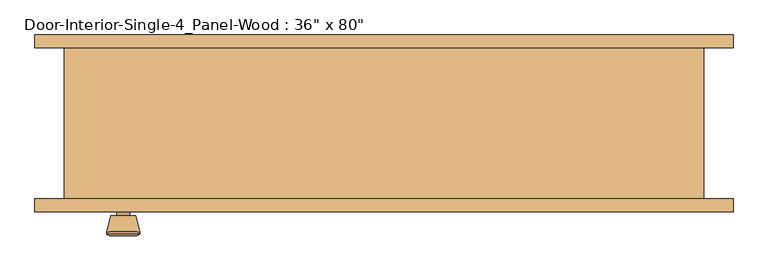
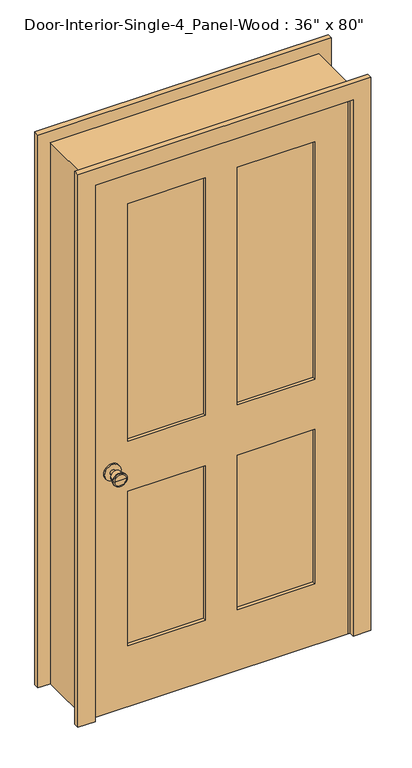
"""IFC4 building model written with IfcOpenShell, lengths in millimetres: door geometry."""

from ifc_helpers import new_model, si_unit, point, frame, frame_2d, origin, place, context, project, spatial, polyline, circle_curve, trimmed, segment, composite_curve, outline, extrude, faceted_brep, source, transform, mapped, element, save
from ifc_brep_helpers import plane_surface, cylinder_surface, revolved_surface, advanced_brep


def door_4c85932b(model_context):
    return source(origin(), model_context, "Body", "SolidModel", [
        advanced_brep(
        [(-393.7, -70.2, 914.4), (-403.7, -70.2, 914.4), (-383.7, -70.2, 914.4), (-373.2241324, -21.2, 914.4), (-414.1758676, -21.2, 914.4), (-393.7, -21.2, 914.4), (-368.7, -23.0278681, 914.4), (-418.7, -23.0278681, 914.4), (-368.7, -26.4915463, 914.4), (-418.7, -26.4915463, 914.4), (-375.063764, -51.2, 914.4), (-412.336236, -51.2, 914.4), (-383.7, -51.2, 914.4), (-403.7, -51.2, 914.4)],
        [
            (0, 1),
            (1, 2, circle_curve(frame((-393.7, -70.2, 914.4), z_axis=(0.0, -1.0, 0.0), x_axis=(-1.0, 0.0, 0.0)), 10.0)),
            (2, 0),
            (2, 1, circle_curve(frame((-393.7, -70.2, 914.4), z_axis=(0.0, -1.0, 0.0), x_axis=(-1.0, 0.0, 0.0)), 10.0)),
            (3, 4, circle_curve(frame((-393.7, -21.2, 914.4), z_axis=(0.0, 1.0, 0.0), x_axis=(-1.0, 0.0, 0.0)), 20.4758676)),
            (4, 5),
            (5, 3),
            (4, 3, circle_curve(frame((-393.7, -21.2, 914.4), z_axis=(0.0, 1.0, 0.0), x_axis=(-1.0, 0.0, 0.0)), 20.4758676)),
            (6, 7, circle_curve(frame((-393.7, -23.0278681, 914.4), z_axis=(0.0, 1.0, 0.0), x_axis=(-1.0, 0.0, 0.0)), 25.0)),
            (7, 4),
            (3, 6),
            (7, 6, circle_curve(frame((-393.7, -23.0278681, 914.4), z_axis=(0.0, 1.0, 0.0), x_axis=(-1.0, 0.0, 0.0)), 25.0)),
            (8, 9, circle_curve(frame((-393.7, -26.4915463, 914.4), z_axis=(0.0, 1.0, 0.0), x_axis=(-1.0, 0.0, 0.0)), 25.0)),
            (9, 7),
            (6, 8),
            (9, 8, circle_curve(frame((-393.7, -26.4915463, 914.4), z_axis=(0.0, 1.0, 0.0), x_axis=(-1.0, 0.0, 0.0)), 25.0)),
            (10, 11, circle_curve(frame((-393.7, -51.2, 914.4), z_axis=(0.0, 1.0, 0.0), x_axis=(-1.0, 0.0, 0.0)), 18.636236)),
            (11, 9),
            (8, 10),
            (11, 10, circle_curve(frame((-393.7, -51.2, 914.4), z_axis=(0.0, 1.0, 0.0), x_axis=(-1.0, 0.0, 0.0)), 18.636236)),
            (12, 13, circle_curve(frame((-393.7, -51.2, 914.4), z_axis=(0.0, 1.0, 0.0), x_axis=(-1.0, 0.0, 0.0)), 10.0)),
            (13, 11),
            (10, 12),
            (13, 12, circle_curve(frame((-393.7, -51.2, 914.4), z_axis=(0.0, 1.0, 0.0), x_axis=(-1.0, 0.0, 0.0)), 10.0)),
            (1, 13),
            (12, 2),
        ],
        [
            plane_surface(frame((-393.7, -70.2, 914.4), z_axis=(0.0, -1.0, 0.0), x_axis=(-1.0, 0.0, 0.0))),
            plane_surface(frame((-393.7, -21.2, 914.4), z_axis=(0.0, 1.0, 0.0), x_axis=(-1.0, 0.0, 0.0))),
            revolved_surface(polyline([(-414.1758676, -21.2, 914.4), (-418.7, -23.0278681, 914.4)]), (-393.7, -70.2, 914.4), (0.0, -1.0, 0.0)),
            cylinder_surface(frame((-393.7, -70.2, 914.4), z_axis=(0.0, -1.0, 0.0), x_axis=(-1.0, 0.0, 0.0)), 25.0),
            revolved_surface(polyline([(-418.7, -26.4915463, 914.4), (-412.336236, -51.2, 914.4)]), (-393.7, -70.2, 914.4), (0.0, -1.0, 0.0)),
            plane_surface(frame((-393.7, -51.2, 914.4), z_axis=(0.0, -1.0, 0.0), x_axis=(-1.0, 0.0, 0.0))),
            cylinder_surface(frame((-393.7, -70.2, 914.4), z_axis=(0.0, -1.0, 0.0), x_axis=(-1.0, 0.0, 0.0)), 10.0),
        ],
        [
            (0, [[1, 2, 3]]),
            (0, [[-3, 4, -1]]),
            (1, [[5, 6, 7]]),
            (1, [[8, -7, -6]]),
            (2, [[9, 10, -5, 11]]),
            (2, [[12, -11, -8, -10]]),
            (3, [[13, 14, -9, 15]]),
            (3, [[16, -15, -12, -14]]),
            (4, [[17, 18, -13, 19]]),
            (4, [[20, -19, -16, -18]]),
            (5, [[21, 22, -17, 23]]),
            (5, [[24, -23, -20, -22]]),
            (6, [[-2, 25, -21, 26]]),
            (6, [[-4, -26, -24, -25]]),
        ],
    ),
        extrude(outline(composite_curve([segment(trimmed(circle_curve(frame_2d((914.4, -393.7)), 30.0), [point((914.4, -423.7))], [point((914.4, -363.7))], False, "CARTESIAN"), True, "CONTINUOUS"), segment(trimmed(circle_curve(frame_2d((914.4, -393.7)), 30.0), [point((914.4, -363.7))], [point((914.4, -423.7))], False, "CARTESIAN"), True, "CONTINUOUS")], self_intersect=False)), frame((0.0, -76.2, 0.0), z_axis=(0.0, 1.0, 0.0), x_axis=(0.0, 0.0, 1.0)), (0.0, 0.0, 1.0), 6.0),
        advanced_brep(
        [(-393.7, -117.125, 914.4), (-383.7, -117.125, 914.4), (-403.7, -117.125, 914.4), (-373.2241324, -166.125, 914.4), (-393.7, -166.125, 914.4), (-414.1758676, -166.125, 914.4), (-368.7, -164.2971319, 914.4), (-418.7, -164.2971319, 914.4), (-368.7, -160.8334537, 914.4), (-418.7, -160.8334537, 914.4), (-375.063764, -136.125, 914.4), (-412.336236, -136.125, 914.4), (-383.7, -136.125, 914.4), (-403.7, -136.125, 914.4)],
        [
            (0, 1),
            (1, 2, circle_curve(frame((-393.7, -117.125, 914.4), z_axis=(0.0, 1.0, 0.0), x_axis=(-1.0, 0.0, 0.0)), 10.0)),
            (2, 0),
            (2, 1, circle_curve(frame((-393.7, -117.125, 914.4), z_axis=(0.0, 1.0, 0.0), x_axis=(-1.0, 0.0, 0.0)), 10.0)),
            (3, 4),
            (4, 5),
            (5, 3, circle_curve(frame((-393.7, -166.125, 914.4), z_axis=(0.0, -1.0, 0.0), x_axis=(-1.0, 0.0, 0.0)), 20.4758676)),
            (3, 5, circle_curve(frame((-393.7, -166.125, 914.4), z_axis=(0.0, -1.0, 0.0), x_axis=(-1.0, 0.0, 0.0)), 20.4758676)),
            (6, 3),
            (5, 7),
            (7, 6, circle_curve(frame((-393.7, -164.2971319, 914.4), z_axis=(0.0, -1.0, 0.0), x_axis=(-1.0, 0.0, 0.0)), 25.0)),
            (6, 7, circle_curve(frame((-393.7, -164.2971319, 914.4), z_axis=(0.0, -1.0, 0.0), x_axis=(-1.0, 0.0, 0.0)), 25.0)),
            (8, 6),
            (7, 9),
            (9, 8, circle_curve(frame((-393.7, -160.8334537, 914.4), z_axis=(0.0, -1.0, 0.0), x_axis=(-1.0, 0.0, 0.0)), 25.0)),
            (8, 9, circle_curve(frame((-393.7, -160.8334537, 914.4), z_axis=(0.0, -1.0, 0.0), x_axis=(-1.0, 0.0, 0.0)), 25.0)),
            (10, 8),
            (9, 11),
            (11, 10, circle_curve(frame((-393.7, -136.125, 914.4), z_axis=(0.0, -1.0, 0.0), x_axis=(-1.0, 0.0, 0.0)), 18.636236)),
            (10, 11, circle_curve(frame((-393.7, -136.125, 914.4), z_axis=(0.0, -1.0, 0.0), x_axis=(-1.0, 0.0, 0.0)), 18.636236)),
            (12, 10),
            (11, 13),
            (13, 12, circle_curve(frame((-393.7, -136.125, 914.4), z_axis=(0.0, -1.0, 0.0), x_axis=(-1.0, 0.0, 0.0)), 10.0)),
            (12, 13, circle_curve(frame((-393.7, -136.125, 914.4), z_axis=(0.0, -1.0, 0.0), x_axis=(-1.0, 0.0, 0.0)), 10.0)),
            (1, 12),
            (13, 2),
        ],
        [
            plane_surface(frame((-393.7, -117.125, 914.4), z_axis=(0.0, 1.0, 0.0), x_axis=(-1.0, 0.0, 0.0))),
            plane_surface(frame((-393.7, -166.125, 914.4), z_axis=(0.0, -1.0, 0.0), x_axis=(-1.0, 0.0, 0.0))),
            revolved_surface(polyline([(-414.1758676, -166.125, 914.4), (-418.7, -164.2971319, 914.4)]), (-393.7, -117.125, 914.4), (0.0, 1.0, 0.0)),
            cylinder_surface(frame((-393.7, -117.125, 914.4), z_axis=(0.0, 1.0, 0.0), x_axis=(-1.0, 0.0, 0.0)), 25.0),
            revolved_surface(polyline([(-418.7, -160.8334537, 914.4), (-412.336236, -136.125, 914.4)]), (-393.7, -117.125, 914.4), (0.0, 1.0, 0.0)),
            plane_surface(frame((-393.7, -136.125, 914.4), z_axis=(0.0, 1.0, 0.0), x_axis=(-1.0, 0.0, 0.0))),
            cylinder_surface(frame((-393.7, -117.125, 914.4), z_axis=(0.0, 1.0, 0.0), x_axis=(-1.0, 0.0, 0.0)), 10.0),
        ],
        [
            (0, [[1, 2, 3]]),
            (0, [[-3, 4, -1]]),
            (1, [[5, 6, 7]]),
            (1, [[-6, -5, 8]]),
            (2, [[9, -7, 10, 11]]),
            (2, [[-10, -8, -9, 12]]),
            (3, [[13, -11, 14, 15]]),
            (3, [[-14, -12, -13, 16]]),
            (4, [[17, -15, 18, 19]]),
            (4, [[-18, -16, -17, 20]]),
            (5, [[21, -19, 22, 23]]),
            (5, [[-22, -20, -21, 24]]),
            (6, [[25, -23, 26, -2]]),
            (6, [[-26, -24, -25, -4]]),
        ],
    ),
        extrude(outline(composite_curve([segment(trimmed(circle_curve(frame_2d((914.4, -393.7)), 30.0), [point((914.4, -423.7))], [point((914.4, -363.7))], False, "CARTESIAN"), True, "CONTINUOUS"), segment(trimmed(circle_curve(frame_2d((914.4, -393.7)), 30.0), [point((914.4, -363.7))], [point((914.4, -423.7))], False, "CARTESIAN"), True, "CONTINUOUS")], self_intersect=False)), frame((0.0, -117.125, 0.0), z_axis=(0.0, 1.0, 0.0), x_axis=(0.0, 0.0, 1.0)), (0.0, 0.0, 1.0), 6.0),
        faceted_brep([(482.6, -111.125, 0.0), (457.2, -111.125, 0.0), (457.2, -76.2, 0.0), (444.5, -76.2, 0.0), (444.5, -41.275, 0.0), (457.2, -41.275, 0.0), (457.2, 117.475, 0.0), (482.6, 117.475, 0.0), (482.6, 117.475, 2057.4), (482.6, -111.125, 2057.4), (457.2, 117.475, 2032.0), (-457.2, 117.475, 2032.0), (-457.2, 117.475, 0.0), (-482.6, 117.475, 0.0), (-482.6, 117.475, 2057.4), (457.2, -41.275, 2032.0), (444.5, -41.275, 2019.3), (-444.5, -41.275, 2019.3), (-444.5, -41.275, 0.0), (-457.2, -41.275, 0.0), (-457.2, -41.275, 2032.0), (444.5, -76.2, 2019.3), (457.2, -76.2, 2032.0), (-457.2, -76.2, 2032.0), (-457.2, -76.2, 0.0), (-444.5, -76.2, 0.0), (-444.5, -76.2, 2019.3), (457.2, -111.125, 2032.0), (-482.6, -111.125, 2057.4), (-482.6, -111.125, 0.0), (-457.2, -111.125, 0.0), (-457.2, -111.125, 2032.0)], [[[0, 1, 2, 3, 4, 5, 6, 7]], [[7, 8, 9, 0]], [[6, 10, 11, 12, 13, 14, 8, 7]], [[5, 15, 10, 6]], [[4, 16, 17, 18, 19, 20, 15, 5]], [[3, 21, 16, 4]], [[2, 22, 23, 24, 25, 26, 21, 3]], [[1, 27, 22, 2]], [[0, 9, 28, 29, 30, 31, 27, 1]], [[8, 14, 28, 9]], [[15, 20, 11, 10]], [[21, 26, 17, 16]], [[27, 31, 23, 22]], [[29, 13, 12, 19, 18, 25, 24, 30]], [[14, 13, 29, 28]], [[20, 19, 12, 11]], [[26, 25, 18, 17]], [[31, 30, 24, 23]]]),
        extrude(outline(polyline([(2032.0, -457.2), (0.0, -457.2), (0.0, 457.2), (2032.0, 457.2), (2032.0, -457.2)]), holes=[polyline([(1912.9375, 57.15), (1912.9375, 336.55), (1009.65, 336.55), (1009.65, 57.15), (1912.9375, 57.15)]), polyline([(1009.65, -57.15), (1009.65, -336.55), (1912.9375, -336.55), (1912.9375, -57.15), (1009.65, -57.15)]), polyline([(819.15, 57.15), (819.15, 336.55), (231.775, 336.55), (231.775, 57.15), (819.15, 57.15)]), polyline([(231.775, -57.15), (231.775, -336.55), (819.15, -336.55), (819.15, -57.15), (231.775, -57.15)])]), frame((0.0, -111.125, 0.0), z_axis=(0.0, 1.0, 0.0), x_axis=(0.0, 0.0, 1.0)), (0.0, 0.0, 1.0), 34.925),
        extrude(outline(polyline([(336.55, -87.8416667), (336.55, -99.4833333), (57.15, -99.4833333), (57.15, -87.8416667), (336.55, -87.8416667)])), frame((0.0, 0.0, 1009.65), z_axis=(0.0, 0.0, 1.0), x_axis=(1.0, 0.0, 0.0)), (0.0, 0.0, 1.0), 903.2875),
        extrude(outline(polyline([(-57.15, -87.8416667), (-57.15, -99.4833333), (-336.55, -99.4833333), (-336.55, -87.8416667), (-57.15, -87.8416667)])), frame((0.0, 0.0, 1009.65), z_axis=(0.0, 0.0, 1.0), x_axis=(1.0, 0.0, 0.0)), (0.0, 0.0, 1.0), 903.2875),
        extrude(outline(polyline([(336.55, -87.8416667), (336.55, -99.4833333), (57.15, -99.4833333), (57.15, -87.8416667), (336.55, -87.8416667)])), frame((0.0, 0.0, 231.775), z_axis=(0.0, 0.0, 1.0), x_axis=(1.0, 0.0, 0.0)), (0.0, 0.0, 1.0), 587.375),
        extrude(outline(polyline([(-57.15, -87.8416667), (-57.15, -99.4833333), (-336.55, -99.4833333), (-336.55, -87.8416667), (-57.15, -87.8416667)])), frame((0.0, 0.0, 231.775), z_axis=(0.0, 0.0, 1.0), x_axis=(1.0, 0.0, 0.0)), (0.0, 0.0, 1.0), 587.375),
        extrude(outline(polyline([(0.0, 527.05), (2101.85, 527.05), (2101.85, -527.05), (0.0, -527.05), (0.0, -463.55), (2038.35, -463.55), (2038.35, 463.55), (0.0, 463.55), (0.0, 527.05)])), frame((0.0, -130.175, 0.0), z_axis=(0.0, 1.0, 0.0), x_axis=(0.0, 0.0, 1.0)), (0.0, 0.0, 1.0), 19.05),
        extrude(outline(polyline([(0.0, 527.05), (2101.85, 527.05), (2101.85, -527.05), (0.0, -527.05), (0.0, -463.55), (2038.35, -463.55), (2038.35, 463.55), (0.0, 463.55), (0.0, 527.05)])), frame((0.0, 117.475, 0.0), z_axis=(0.0, 1.0, 0.0), x_axis=(0.0, 0.0, 1.0)), (0.0, 0.0, 1.0), 19.05),
    ])


if __name__ == "__main__":
    model = new_model("IFC4")
    model_context = context("Model", 3, world=origin())
    ifc_project = project(units=[si_unit("LENGTHUNIT", "METRE", prefix="MILLI")], contexts=[model_context])
    site = spatial("IfcSite", under=ifc_project)
    building = spatial("IfcBuilding", under=site)
    placement = place(None, origin())
    door_shape = door_4c85932b(model_context)
    element("IfcDoor", 1, ObjectType="Door-Interior-Single-4_Panel-Wood : 36\" x 80\"", at=placement, inside=building, context=model_context, shape_type="MappedRepresentation", body=[
        mapped(door_shape, transform((0.0, 0.0, 0.0), x_axis=(1.0, 0.0, 0.0), y_axis=(0.0, 1.0, 0.0), z_axis=(0.0, 0.0, 1.0))),
    ])
    save(model, "model.ifc")

# Revit data of these elements
# Type "Door-Interior-Single-4_Panel-Wood : 36\" x 80\""
#   Type Mark = "9"
#   Assembly Code = "C1020300"
#   Analytic Construction = "Wooden"
#   Top Rail = 0' - 4 11/16"
#   Thickness = 0' - 1 3/8"
#   Thermal Resistance (R) = 2.5876 (h·ft²·°F)/BTU
#   Swing Angle [instance default] = 90.00°
#   Stiles = 0' - 4 3/4"
#   Rough Width = 3' - 2"
#   Rough Height = 6' - 9"
#   Mullion = 0' - 4 1/2"
#   Lock Rail = 0' - 7 1/2"
#   Height = 6' - 8"
#   Width = 3' - 0"
#   Heat Transfer Coefficient (U) = 0.3865 BTU/(h·ft²·°F)
#   Bottom Rail = 0' - 9 1/8"
#   Trim Material = Cherry
#   Panel Material = Cherry
#   Frame Material = Cherry
#   Door Handle Material = Aluminum
#   Visual Light Transmittance = 0
#   Solar Heat Gain Coefficient = 0
#   Wall Closure = (empty or 0)
#   Function = (empty or 0)
# Element 1 (IfcDoor, "Door-Interior-Single-4_Panel-Wood : 36\" x 80\"")
#   Materials on its faces: "Cherry", "Aluminum"
# Materials
#   "Cherry": class "Wood", colour RGB 226 177 128, transparency 0, Description = "Prunus Serotina", Cost = 0
#   "Aluminum": class "Metal", colour RGB 247 247 247, transparency 0, Description = "Aluminum 6061", Cost = 0
